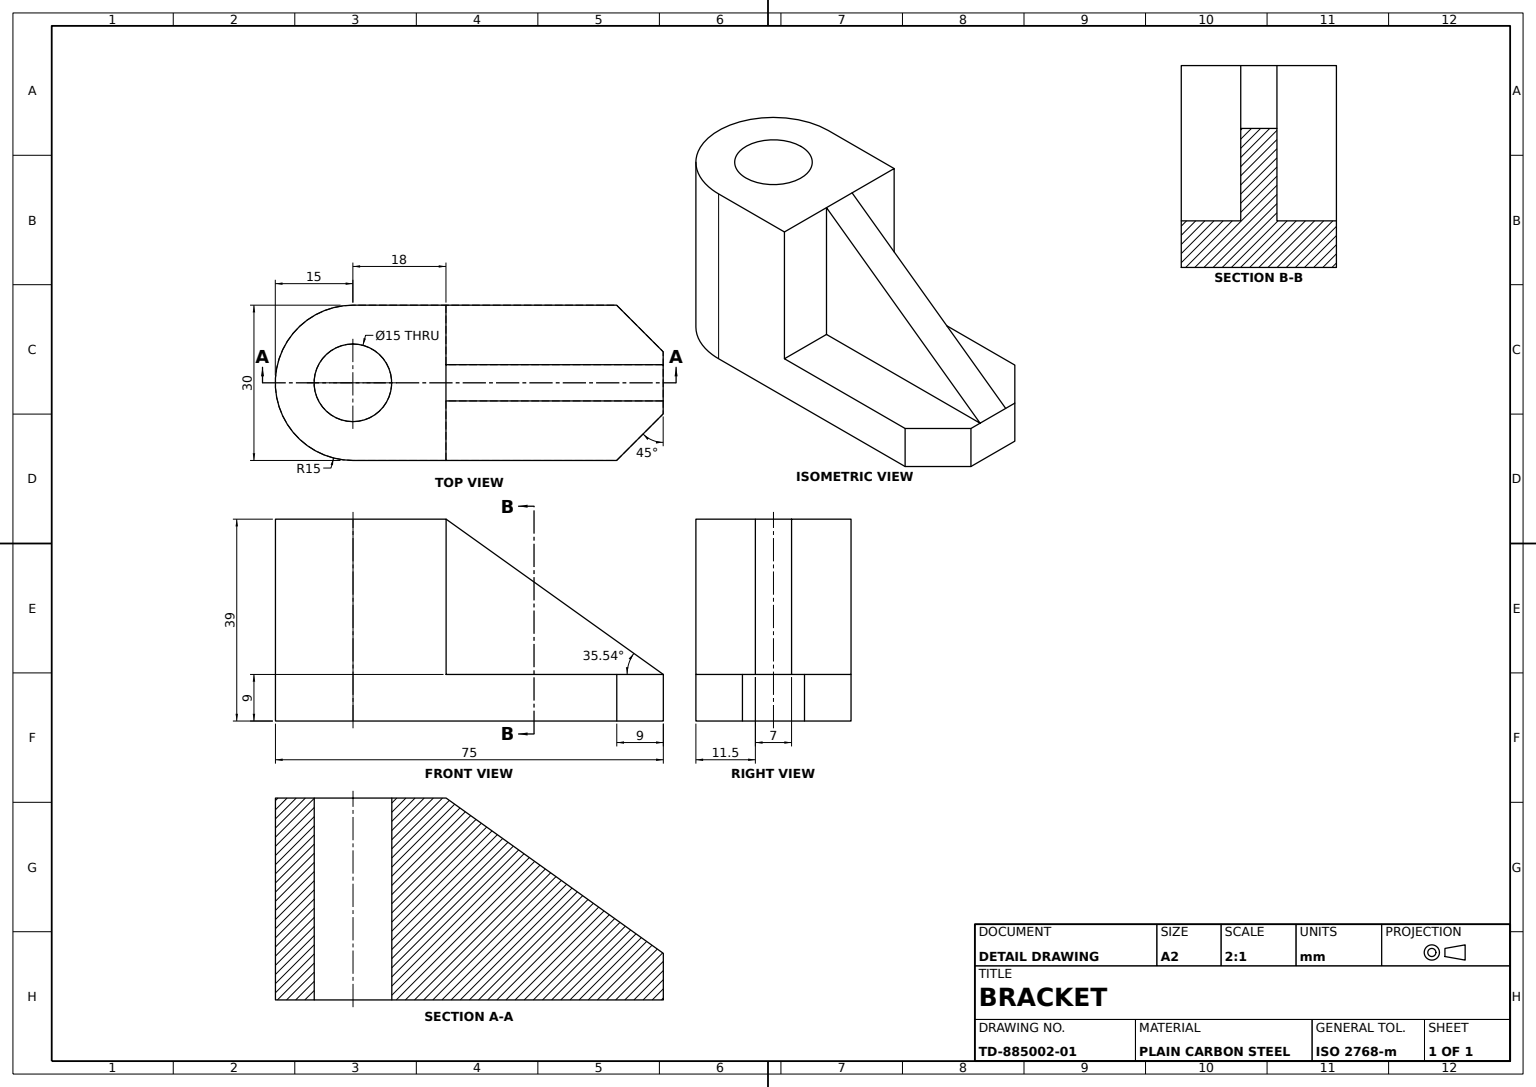
SolidWorks part; units mm, degrees
material "Plain Carbon Steel"
ref_plane "Front Plane" through (0, 0, 0) normal (0, 0, 1) x (1, 0, 0)
ref_plane "Top Plane" through (0, 0, 0) normal (0, 1, 0) x (1, 0, 0)
ref_plane "Right Plane" through (0, 0, 0) normal (1, 0, 0) x (0, 0, -1)
sketch "Base Plate Sketch" plane through (0, 0, 0) normal (0, 1, 0) x (1, 0, 0)
  line L0 (28.5, 15) -> (37.5, 6)
  line L1 (-37.5, 15) -> (28.5, 15)
  line L2 (-37.5, 15) -> (-37.5, -15)
  line L3 (-37.5, -15) -> (28.5, -15)
  line L4 (37.5, 6) -> (37.5, -6)
  line L5 (-37.5, 15) -> (37.5, -15) construction
  line L6 (-37.5, -15) -> (37.5, 15) construction
  line L7 (37.5, -6) -> (28.5, -15)
  point P0 (0, 0)
  dimension "D1" = 75
  dimension "D2" = 30
extrude "Base Plate" add sketch "Base Plate Sketch" along normal blind 9
sketch "Base End Cut Sketch" plane through (0, 9, 0) normal (0, 1, 0) x (1, 0, 0)
  line L0 (-37.5, -15) -> (-22.5, -15)
  line L1 (-37.5, -15) -> (28.5, -15) construction
  line L2 (-22.5, -15) -> (-22.5, 15) construction
  line L3 (-22.5, 15) -> (-37.5, 15)
  line L5 (-37.5, 15) -> (-37.5, -15)
  line L6 (-37.5, -15) -> (-22.5, -15)
  arc A0 (-22.5, 15) -> (-22.5, -15) centre (-22.5, 0) ccw
  line M4 (-37.5, 15) -> (-37.5, -15)
  line M5 (-37.5, -15) -> (28.5, -15)
  line M9 (28.5, 15) -> (-37.5, 15)
  dimension "D2" = 30
  dimension "D1" = 15
extrude "Base End Cut" cut sketch "Base End Cut Sketch" against normal blind 9 contours A0 L5 M5 | A0 M9 M4
sketch "Upright Boss Sketch" plane through (0, 9, 0) normal (0, 1, 0) x (1, 0, 0)
  line L0 (-22.5, 15) -> (-4.5, 15)
  line L1 (-4.5, 15) -> (-4.5, -15)
  line L2 (-4.5, -15) -> (-22.5, -15)
  line L5 (28.5, 15) -> (-22.5, 15)
  line L6 (-22.5, -15) -> (28.5, -15)
  line L7 (28.5, -15) -> (37.5, -6)
  line L8 (37.5, -6) -> (37.5, 6)
  line L9 (37.5, 6) -> (28.5, 15)
  line L10 (-4.5, 15) -> (-22.5, 15)
  line L11 (-22.5, -15) -> (-4.5, -15)
  circle A0 centre (-22.5, 0) radius 7.5
  arc A1 (-22.5, 15) -> (-22.5, -15) centre (-22.5, 0) ccw
  arc A2 (-22.5, 15) -> (-22.5, -15) centre (-22.5, 0) ccw
  line M8 (28.5, 15) -> (-22.5, 15)
  arc M9 (-22.5, 15) -> (-22.5, -15) centre (-22.5, 0) ccw
  line M10 (-22.5, -15) -> (28.5, -15)
  dimension "D3" = 15
  dimension "D2" = 18
  dimension "D1" = 0
extrude "Upright Boss" add sketch "Upright Boss Sketch" along normal blind 30 contours L1 A0 M8 M9 M10
sketch "Support Rib Sketch" plane through (0, 0, 0) normal (0, 0, 1) x (1, 0, 0)
  line L0 (-4.5, 39) -> (37.5, 9)
  line L1 (37.5, 9) -> (-4.5, 9)
  line L2 (-4.5, 9) -> (-4.5, 39)
extrude "Support Rib" add sketch "Support Rib Sketch" along normal mid plane 7
sketch "Boss Bore Sketch" plane through (0, 39, 0) normal (0, 1, 0) x (1, 0, 0)
  circle A0 centre (-22.5, 0) radius 7.5 construction
  circle A1 centre (-22.5, 0) radius 7.5
extrude "Boss Bore" cut sketch "Boss Bore Sketch" against normal through all
